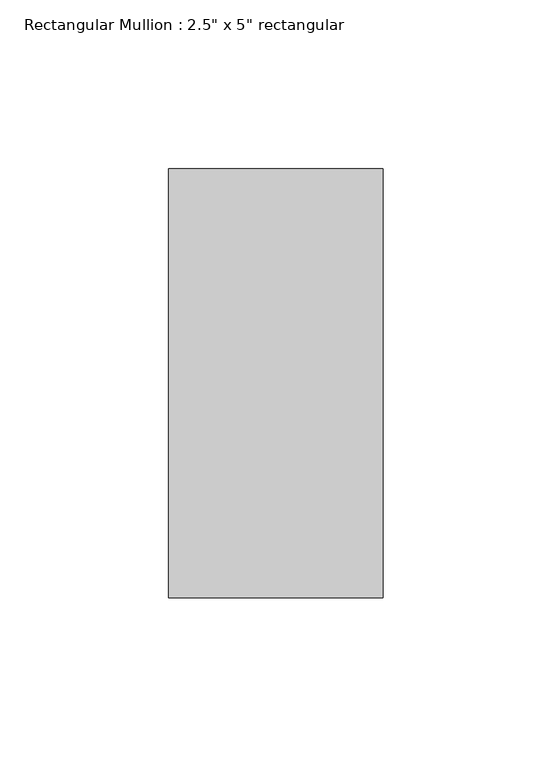
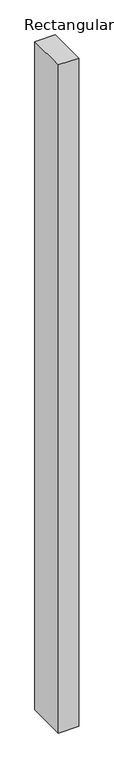
"""IFC4 building model written with IfcOpenShell, lengths in millimetres: member geometry."""

from ifc_helpers import new_model, si_unit, frame, origin, place, context, project, spatial, polyline, outline, extrude, source, transform, mapped, element, save


def member_1182c56c(model_context):
    return source(origin(), model_context, "Body", "SweptSolid", [
        extrude(outline(polyline([(31.75, 63.5), (31.75, -63.5), (-31.75, -63.5), (-31.75, 63.5), (31.75, 63.5)])), frame((0.0, 0.0, -2209.8), z_axis=(0.0, 0.0, 1.0), x_axis=(1.0, 0.0, 0.0)), (0.0, 0.0, 1.0), 2209.8),
    ])


if __name__ == "__main__":
    model = new_model("IFC4")
    model_context = context("Model", 3, world=origin())
    ifc_project = project(units=[si_unit("LENGTHUNIT", "METRE", prefix="MILLI")], contexts=[model_context])
    site = spatial("IfcSite", under=ifc_project)
    building = spatial("IfcBuilding", under=site)
    placement = place(None, origin())
    member_shape = member_1182c56c(model_context)
    element("IfcMember", 1, ObjectType="Rectangular Mullion : 2.5\" x 5\" rectangular", at=placement, inside=building, context=model_context, shape_type="MappedRepresentation", body=[
        mapped(member_shape, transform((0.0, 0.0, 0.0), x_axis=(1.0, 0.0, 0.0), y_axis=(0.0, 1.0, 0.0), z_axis=(0.0, 0.0, 1.0))),
    ])
    save(model, "model.ifc")

# Revit data of these elements
# Type "Rectangular Mullion : 2.5\" x 5\" rectangular"
#   built-in parameter 1007304 = 0.416667 (stored number, unit not read)
#   built-in parameter 1007301 = 0.104167 (stored number, unit not read)
#   built-in parameter 1007300 = 0.104167 (stored number, unit not read)
# Element 1 (IfcMember, "Rectangular Mullion : 2.5\" x 5\" rectangular")
#   Materials on its faces: "Aluminum"
# Materials
#   "Aluminum": class "Metal", colour RGB 247 247 247, transparency 0, Description = "Aluminum 6061", Cost = 0
